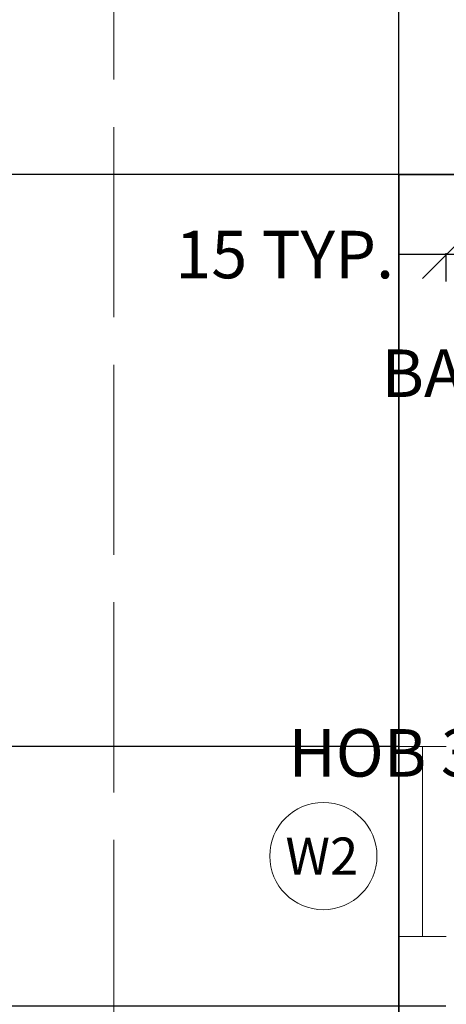
# Model space of a CAD drawing. Units: inches. Extents: x -1198 to -69, y -512 to 437.
# Tile 5 of 50: x -1067 to -1013, y 158 to 283. Entities that reach past the tile are written whole.
import ezdxf

# ---------------------------------------------------------------- set-up
doc = ezdxf.new("R2010")
doc.units = ezdxf.units.IN
doc.header["$MEASUREMENT"] = 0
doc.linetypes.add('ACAD_ISO02W100', pattern=[15, 12, -3])
for name, color, linetype, lineweight in [('A-ANNO-DIMS', 2, 'Continuous', 18), ('A-ANNO-SYMB', 7, 'Continuous', 18), ('A-WALL', 7, 'Continuous', 35), ('C-PROP', 141, 'ACAD_ISO02W100', 18), ('windows', 160, 'Continuous', 18)]:
    doc.layers.add(name, color=color, linetype=linetype, lineweight=lineweight)
doc.styles.get("Standard").update_dxf_attribs({"font": 'arial.ttf'})
doc.dimstyles.get("Standard").update_dxf_attribs({"dimtxt": 6, "dimasz": 6, "dimexe": 0.18, "dimexo": 0.0625, "dimgap": 0.09, "dimtad": 0, "dimtih": 1, "dimtoh": 1, "dimdec": 0, "dimzin": 0, "dimdsep": 46, "dimlunit": 4, "dimtxsty": 'Standard', "dimblk": 'OBLIQUE', "dimcen": 0.09, "dimadec": 0, "dimazin": 0, "dimtfac": 1, "dimtdec": 0, "dimtofl": 0, "dimtmove": 0, "dimatfit": 3, "dimfxl": 1, "dimtolj": 1, "dimtzin": 0, "dimarcsym": 0})

# ---------------------------------------------------------------- blocks, each defined once
blk = doc.blocks.new('WIN-W2-24')
at = {"ltscale": 10}
for p, q in [((0, 6), (0, 0)), ((24, 6), (24, 0)), ((0, 3), (24, 3))]:
    blk.add_line(p, q, dxfattribs=at)
blk = doc.blocks.new('TAG-W2')
at = {"ltscale": 10}
blk.add_circle((0, 0), 6.77, dxfattribs=at)
blk.add_text('W2', height=4.7, dxfattribs=at).set_placement((-4.79, -2.36))
blk = doc.blocks.new('_Oblique')
at = {"color": 0, "linetype": 'ByBlock', "lineweight": -2}
blk.add_line((-0.5, -0.5), (0.5, 0.5), dxfattribs=at)
blk = doc.blocks.new('*D40')
at = {"layer": 'A-ANNO-DIMS', "color": 0, "lineweight": -2, "ltscale": 10, "transparency": 16777216}
for p, q in [((-997.84, 249.67), (-994.26, 249.67)), ((-994.44, 249.67), (-994.44, 241.34)), ((-994.44, 226.62), (-994.44, 234.95)), ((-997.84, 226.62), (-994.26, 226.62))]:
    blk.add_line(p, q, dxfattribs=at)
at = {"layer": 'DEFPOINTS', "color": 0, "ltscale": 10, "transparency": 16777216}
for p in [(-997.9, 249.67), (-994.44, 249.67), (-997.9, 226.62)]:
    blk.add_point(p, dxfattribs=at)
at = {"layer": 'A-ANNO-DIMS', "color": 0, "lineweight": -2, "ltscale": 10, "transparency": 16777216, "xscale": 6, "yscale": 6, "zscale": 6}
for p, rotation in [((-994.44, 249.67), 90), ((-994.44, 226.62), 270)]:
    blk.add_blockref('_Oblique', p, dxfattribs=dict(at, rotation=rotation))
at = {"layer": 'A-ANNO-DIMS', "color": 0, "ltscale": 10, "transparency": 16777216, "insert": (-994.44, 238.15), "char_height": 6, "attachment_point": 5}
blk.add_mtext('\\A1;BASIN 23 TYP.', dxfattribs=at)
blk = doc.blocks.new('*D41')
at = {"layer": 'A-ANNO-DIMS', "color": 0, "lineweight": -2, "ltscale": 10, "transparency": 16777216}
for p, q in [((-1012.75, 253.13), (-1018.75, 253.13)), ((-1012.75, 249.73), (-1012.75, 253.31)), ((-997.9, 253.13), (-1012.75, 253.13)), ((-997.9, 249.73), (-997.9, 253.31))]:
    blk.add_line(p, q, dxfattribs=at)
at = {"layer": 'DEFPOINTS', "color": 0, "ltscale": 10, "transparency": 16777216}
for p in [(-1012.75, 253.13), (-1012.75, 249.67), (-997.9, 249.67)]:
    blk.add_point(p, dxfattribs=at)
at = {"layer": 'A-ANNO-DIMS', "color": 0, "lineweight": -2, "ltscale": 10, "transparency": 16777216, "xscale": 6, "yscale": 6, "zscale": 6, "rotation": 180}
blk.add_blockref('_Oblique', (-1012.75, 253.13), dxfattribs=at)
at = {"layer": 'A-ANNO-DIMS', "color": 0, "lineweight": -2, "ltscale": 10, "transparency": 16777216, "xscale": 6, "yscale": 6, "zscale": 6}
blk.add_blockref('_Oblique', (-997.9, 253.13), dxfattribs=at)
at = {"layer": 'A-ANNO-DIMS', "color": 0, "ltscale": 10, "transparency": 16777216, "insert": (-1033.16, 253.13), "char_height": 6, "attachment_point": 5}
blk.add_mtext('\\A1;15 TYP.', dxfattribs=at)
blk = doc.blocks.new('*D50')
at = {"layer": 'A-ANNO-DIMS', "color": 0, "lineweight": -2, "ltscale": 10, "transparency": 16777216}
for p, q in [((-978.46, 190.22), (-984.46, 190.22)), ((-978.46, 185.29), (-978.46, 190.4)), ((-945.16, 190.22), (-978.46, 190.22)), ((-945.16, 185.29), (-945.16, 190.4))]:
    blk.add_line(p, q, dxfattribs=at)
at = {"layer": 'DEFPOINTS', "color": 0, "ltscale": 10, "transparency": 16777216}
for p in [(-978.46, 190.22), (-978.46, 185.23), (-945.16, 185.23)]:
    blk.add_point(p, dxfattribs=at)
at = {"layer": 'A-ANNO-DIMS', "color": 0, "lineweight": -2, "ltscale": 10, "transparency": 16777216, "xscale": 6, "yscale": 6, "zscale": 6, "rotation": 180}
blk.add_blockref('_Oblique', (-978.46, 190.22), dxfattribs=at)
at = {"layer": 'A-ANNO-DIMS', "color": 0, "lineweight": -2, "ltscale": 10, "transparency": 16777216, "xscale": 6, "yscale": 6, "zscale": 6}
blk.add_blockref('_Oblique', (-945.16, 190.22), dxfattribs=at)
at = {"layer": 'A-ANNO-DIMS', "color": 0, "ltscale": 10, "transparency": 16777216, "insert": (-1009.24, 190.22), "char_height": 6, "attachment_point": 5}
blk.add_mtext('\\A1;HOB 33 TYP.', dxfattribs=at)
blk = doc.blocks.new('*D61')
at = {"layer": 'A-ANNO-DIMS', "color": 0, "lineweight": -2, "ltscale": 10, "transparency": 16777216}
for p, q in [((-1054.81, 299.23), (-1188.2, 299.23)), ((-1188.02, 299.23), (-1188.02, 20.38)), ((-1188.02, -264.77), (-1188.02, 14.07)), ((-1054.81, -264.77), (-1188.2, -264.77))]:
    blk.add_line(p, q, dxfattribs=at)
at = {"layer": 'DEFPOINTS', "color": 0, "ltscale": 10, "transparency": 16777216}
for p in [(-1054.75, 299.23), (-1188.02, -264.77), (-1054.75, -264.77)]:
    blk.add_point(p, dxfattribs=at)
at = {"layer": 'A-ANNO-DIMS', "color": 0, "lineweight": -2, "ltscale": 10, "transparency": 16777216, "xscale": 6, "yscale": 6, "zscale": 6}
for p, rotation in [((-1188.02, 299.23), 90), ((-1188.02, -264.77), 270)]:
    blk.add_blockref('_Oblique', p, dxfattribs=dict(at, rotation=rotation))
at = {"layer": 'A-ANNO-DIMS', "color": 0, "ltscale": 10, "transparency": 16777216, "insert": (-1188.02, 17.23), "char_height": 6, "attachment_point": 5}
blk.add_mtext('\\A1;564', dxfattribs=at)
blk = doc.blocks.new('*D65')
at = {"layer": 'A-ANNO-DIMS', "color": 0, "lineweight": -2, "ltscale": 10, "transparency": 16777216}
for p, q in [((-1054.75, 299.29), (-1054.75, 433.18)), ((-1054.75, 433), (-1041.13, 433)), ((-1018.75, 433), (-1032.37, 433)), ((-1018.75, 263.29), (-1018.75, 433.18))]:
    blk.add_line(p, q, dxfattribs=at)
at = {"layer": 'DEFPOINTS', "color": 0, "ltscale": 10, "transparency": 16777216}
for p in [(-1018.75, 433), (-1054.75, 299.23), (-1018.75, 263.23)]:
    blk.add_point(p, dxfattribs=at)
at = {"layer": 'A-ANNO-DIMS', "color": 0, "lineweight": -2, "ltscale": 10, "transparency": 16777216, "xscale": 6, "yscale": 6, "zscale": 6, "rotation": 180}
blk.add_blockref('_Oblique', (-1054.75, 433), dxfattribs=at)
at = {"layer": 'A-ANNO-DIMS', "color": 0, "lineweight": -2, "ltscale": 10, "transparency": 16777216, "xscale": 6, "yscale": 6, "zscale": 6}
blk.add_blockref('_Oblique', (-1018.75, 433), dxfattribs=at)
at = {"layer": 'A-ANNO-DIMS', "color": 0, "ltscale": 10, "transparency": 16777216, "insert": (-1036.75, 433), "char_height": 6, "attachment_point": 5}
blk.add_mtext('\\A1;36', dxfattribs=at)
blk = doc.blocks.new('*D78')
at = {"layer": 'A-ANNO-DIMS', "color": 0, "lineweight": -2, "ltscale": 10, "transparency": 16777216}
for p, q in [((-1018.75, 263.29), (-1018.75, 433.18)), ((-1018.75, 433), (-997.39, 433)), ((-955.56, 433), (-976.92, 433)), ((-955.56, 263.29), (-955.56, 433.18))]:
    blk.add_line(p, q, dxfattribs=at)
at = {"layer": 'DEFPOINTS', "color": 0, "ltscale": 10, "transparency": 16777216}
for p in [(-955.56, 433), (-1018.75, 263.23), (-955.56, 263.23)]:
    blk.add_point(p, dxfattribs=at)
at = {"layer": 'A-ANNO-DIMS', "color": 0, "lineweight": -2, "ltscale": 10, "transparency": 16777216, "xscale": 6, "yscale": 6, "zscale": 6, "rotation": 180}
blk.add_blockref('_Oblique', (-1018.75, 433), dxfattribs=at)
at = {"layer": 'A-ANNO-DIMS', "color": 0, "lineweight": -2, "ltscale": 10, "transparency": 16777216, "xscale": 6, "yscale": 6, "zscale": 6}
blk.add_blockref('_Oblique', (-955.56, 433), dxfattribs=at)
at = {"layer": 'A-ANNO-DIMS', "color": 0, "ltscale": 10, "transparency": 16777216, "insert": (-987.16, 433), "char_height": 6, "attachment_point": 5}
blk.add_mtext('\\A1;63.19', dxfattribs=at)
blk = doc.blocks.new('*D80')
at = {"layer": 'A-ANNO-DIMS', "color": 0, "lineweight": -2, "ltscale": 10, "transparency": 16777216}
for p, q in [((-1012.81, 158.23), (-1188.2, 158.23)), ((-1188.02, 158.23), (-1188.02, 140.33)), ((-1188.02, 116.23), (-1188.02, 134.13)), ((-1018.81, 116.23), (-1188.2, 116.23))]:
    blk.add_line(p, q, dxfattribs=at)
at = {"layer": 'DEFPOINTS', "color": 0, "ltscale": 10, "transparency": 16777216}
for p in [(-1188.02, 158.23), (-1012.75, 158.23), (-1018.75, 116.23)]:
    blk.add_point(p, dxfattribs=at)
at = {"layer": 'A-ANNO-DIMS', "color": 0, "lineweight": -2, "ltscale": 10, "transparency": 16777216, "xscale": 6, "yscale": 6, "zscale": 6}
for p, rotation in [((-1188.02, 158.23), 90), ((-1188.02, 116.23), 270)]:
    blk.add_blockref('_Oblique', p, dxfattribs=dict(at, rotation=rotation))
at = {"layer": 'A-ANNO-DIMS', "color": 0, "ltscale": 10, "transparency": 16777216, "insert": (-1188.02, 137.23), "char_height": 6, "attachment_point": 5}
blk.add_mtext('\\A1;42', dxfattribs=at)
blk = doc.blocks.new('*D81')
at = {"layer": 'A-ANNO-DIMS', "color": 0, "lineweight": -2, "ltscale": 10, "transparency": 16777216}
for p, q in [((-1018.81, 263.23), (-1188.2, 263.23)), ((-1188.02, 263.23), (-1188.02, 230.23)), ((-1188.02, 191.02), (-1188.02, 224.02)), ((-1018.81, 191.02), (-1188.2, 191.02))]:
    blk.add_line(p, q, dxfattribs=at)
at = {"layer": 'DEFPOINTS', "color": 0, "ltscale": 10, "transparency": 16777216}
for p in [(-1188.02, 263.23), (-1018.75, 263.23), (-1018.75, 191.02)]:
    blk.add_point(p, dxfattribs=at)
at = {"layer": 'A-ANNO-DIMS', "color": 0, "lineweight": -2, "ltscale": 10, "transparency": 16777216, "xscale": 6, "yscale": 6, "zscale": 6}
for p, rotation in [((-1188.02, 263.23), 90), ((-1188.02, 191.02), 270)]:
    blk.add_blockref('_Oblique', p, dxfattribs=dict(at, rotation=rotation))
at = {"layer": 'A-ANNO-DIMS', "color": 0, "ltscale": 10, "transparency": 16777216, "insert": (-1188.02, 227.12), "char_height": 6, "attachment_point": 5}
blk.add_mtext('\\A1;72.2', dxfattribs=at)

msp = doc.modelspace()

# ---------------------------------------------------------------- linework, layer by layer
at = {"layer": 'A-WALL', "ltscale": 10}
for p, q in [((-697.7509, 263.2277), (-1018.7509, 263.2277)), ((-1018.7509, 263.2277), (-1018.7509, -228.7723))]:
    msp.add_line(p, q, dxfattribs=at)
at = {"layer": 'C-PROP', "ltscale": 2}
msp.add_lwpolyline([(-1054.7509, 299.2277), (-334.7509, 299.2277), (-334.7509, -264.7723), (-1054.7509, -264.7723)], close=True, dxfattribs=at)

# ---------------------------------------------------------------- block references
at = {"layer": 'A-ANNO-SYMB'}
msp.add_blockref('TAG-W2', (-1028.2781, 177.1933), dxfattribs=at)
at = {"layer": 'windows', "rotation": 89.99999999999928}
msp.add_blockref('WIN-W2-24', (-1012.7512, 167.0213), dxfattribs=at)

# ---------------------------------------------------------------- dimensions: what is measured, and where the dimension line sits
at = {"layer": 'A-ANNO-DIMS', "ltscale": 10}
for base, p1, p2, override, picture, middle in [((-1018.7509, 433.0036), (-1054.7509, 299.2277), (-1018.7509, 263.2277), {"dimdec": 0, "dimlfac": 1, "dimrnd": 0, "dimzin": 0, "dimdsep": 46, "dimlunit": 2}, '*D65', (-1036.7509, 433.0036)), ((-955.5591, 433.0036), (-1018.7509, 263.2277), (-955.5591, 263.2277), {"dimdec": 2, "dimlfac": 1, "dimrnd": 0, "dimzin": 0, "dimdsep": 46, "dimlunit": 2}, '*D78', (-987.155, 433.0036))]:
    dim = msp.add_linear_dim(base=base, p1=p1, p2=p2, dimstyle='Standard', override=override, dxfattribs=at)
    dim.commit()
    dim.dimension.update_dxf_attribs({"geometry": picture, "text_midpoint": middle})
for base, p1, p2, override, picture, middle in [((-1188.0248, -264.7723), (-1054.7509, 299.2277), (-1054.7509, -264.7723), {"dimdec": 0, "dimlfac": 1, "dimrnd": 0, "dimzin": 0, "dimdsep": 46, "dimlunit": 2}, '*D61', (-1188.0248, 17.2277)), ((-1188.0248, 263.2277), (-1018.7509, 191.0212), (-1018.7509, 263.2277), {"dimdec": 1, "dimlfac": 1, "dimrnd": 0, "dimzin": 0, "dimdsep": 46, "dimlunit": 2}, '*D81', (-1188.0248, 227.1244)), ((-1188.0248, 158.2277), (-1018.7509, 116.2277), (-1012.7509, 158.2277), {"dimdec": 0, "dimlfac": 1, "dimrnd": 0, "dimzin": 0, "dimdsep": 46, "dimlunit": 2}, '*D80', (-1188.0248, 137.2277))]:
    dim = msp.add_linear_dim(base=base, p1=p1, p2=p2, angle=90, dimstyle='Standard', override=override, dxfattribs=at)
    dim.commit()
    dim.dimension.update_dxf_attribs({"geometry": picture, "text_midpoint": middle})
for base, p1, p2, angle, text, picture, middle in [((-1012.7509, 253.1284), (-997.9022, 249.6708), (-1012.7509, 249.6708), 180, '<> TYP.', '*D41', (-1033.1615, 253.1284)), ((-994.4446, 249.6708), (-997.9022, 226.6201), (-997.9022, 249.6708), 90, 'BASIN <> TYP.', '*D40', (-994.4446, 238.1454)), ((-978.4621, 190.2226), (-945.1627, 185.2277), (-978.4621, 185.2277), 180, 'HOB <> TYP.', '*D50', (-1009.2397, 190.2226))]:
    dim = msp.add_linear_dim(base=base, p1=p1, p2=p2, angle=angle, text=text, dimstyle='Standard', override={"dimdec": 0, "dimlfac": 1, "dimrnd": 0, "dimzin": 0, "dimdsep": 46, "dimlunit": 2}, dxfattribs=at)
    dim.commit()
    dim.dimension.update_dxf_attribs({"geometry": picture, "text_midpoint": middle})

doc.saveas('drawing.dxf')
